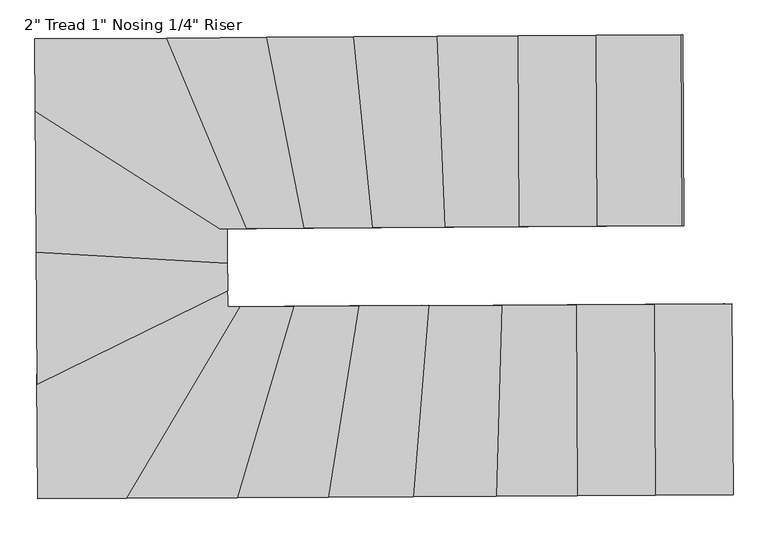
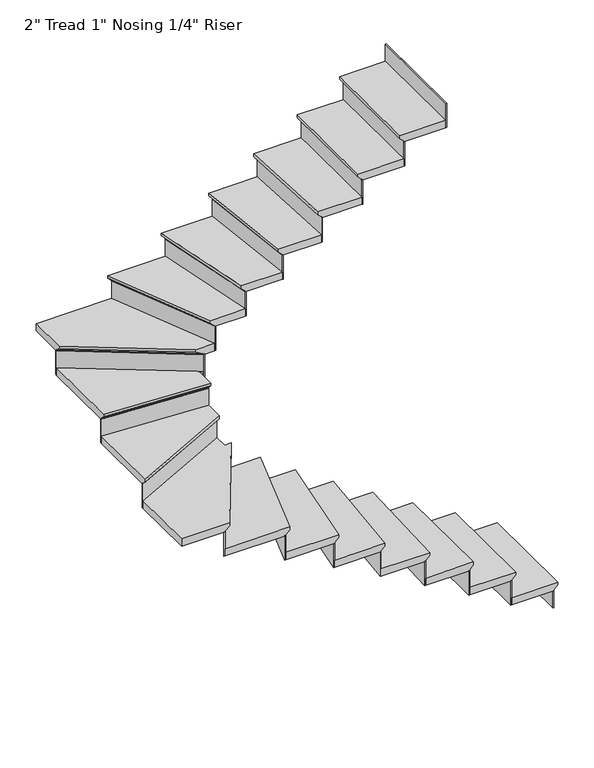
"""IFC4 building model written with IfcOpenShell, lengths in millimetres: stair flight geometry."""

from ifc_helpers import new_model, si_unit, origin, place, context, project, spatial, faceted_brep, source, transform, mapped, element, save


def stair_flight_c1b2dc12(model_context):
    return source(origin(), model_context, "Body", "Brep", [
        faceted_brep([(-120.6930289, -3539.621908, 12951.8833333), (-120.6930289, -3539.621908, 12970.9333333), (-116.4891496, -4225.4090232, 12970.9333333), (-116.4891496, -4225.4090232, 12951.8833333), (-146.0925517, -3539.7776072, 12926.4833333), (-141.8886723, -4225.5647224, 12926.4833333), (-425.4873024, -3541.4902988, 12970.9333333), (-421.283423, -4227.277414, 12970.9333333), (-141.8886723, -4225.5647224, 12920.1333333), (-421.283423, -4227.277414, 12920.1333333), (-425.4873024, -3541.4902988, 12920.1333333), (-146.0925517, -3539.7776072, 12920.1333333)], [[[0, 1, 2, 3]], [[4, 0, 3, 5]], [[2, 1, 6, 7]], [[8, 9, 10, 11]], [[2, 7, 9, 8, 5, 3]], [[8, 11, 4, 5]], [[6, 1, 0, 4, 11, 10]], [[7, 6, 10, 9]]]),
        faceted_brep([(-146.0925517, -3539.7776072, 12920.1333333), (-146.0925517, -3539.7776072, 12801.6), (-152.4424324, -3539.816532, 12801.6), (-152.4424324, -3539.816532, 12920.1333333), (-141.8886723, -4225.5647224, 12920.1333333), (-148.238553, -4225.6036472, 12920.1333333), (-148.238553, -4225.6036472, 12801.6), (-141.8886723, -4225.5647224, 12801.6)], [[[0, 1, 2, 3]], [[4, 5, 6, 7]], [[1, 0, 4, 7]], [[2, 1, 7, 6]], [[3, 2, 6, 5]], [[0, 3, 5, 4]]]),
        faceted_brep([(-425.4873024, -3541.4902988, 13089.4666667), (-425.4873024, -3541.4902988, 12920.1333333), (-431.8371831, -3541.5292236, 12920.1333333), (-431.8371831, -3541.5292236, 13089.4666667), (-421.283423, -4227.277414, 13089.4666667), (-427.6333037, -4227.3163388, 13089.4666667), (-427.6333037, -4227.3163388, 12920.1333333), (-421.283423, -4227.277414, 12920.1333333)], [[[0, 1, 2, 3]], [[4, 5, 6, 7]], [[1, 0, 4, 7]], [[2, 1, 7, 6]], [[3, 2, 6, 5]], [[0, 3, 5, 4]]]),
        faceted_brep([(-395.8839002, -4227.1217148, 13140.2666667), (-400.0877796, -3541.3345996, 13140.2666667), (-704.882053, -3543.2029904, 13140.2666667), (-700.6781736, -4228.9901056, 13140.2666667), (-421.283423, -4227.277414, 13089.4666667), (-700.6781736, -4228.9901056, 13089.4666667), (-704.882053, -3543.2029904, 13089.4666667), (-425.4873024, -3541.4902988, 13089.4666667), (-421.283423, -4227.277414, 13095.8166667), (-395.8839002, -4227.1217148, 13121.2166667), (-425.4873024, -3541.4902988, 13095.8166667), (-400.0877796, -3541.3345996, 13121.2166667)], [[[0, 1, 2, 3]], [[4, 5, 6, 7]], [[0, 3, 5, 4, 8, 9]], [[4, 7, 10, 8]], [[2, 1, 11, 10, 7, 6]], [[3, 2, 6, 5]], [[11, 1, 0, 9]], [[10, 11, 9, 8]]]),
        faceted_brep([(-704.882053, -3543.2029904, 13258.8), (-704.882053, -3543.2029904, 13089.4666667), (-711.2319337, -3543.2419152, 13089.4666667), (-711.2319337, -3543.2419152, 13258.8), (-700.6781736, -4228.9901056, 13258.8), (-707.0280543, -4229.0290304, 13258.8), (-707.0280543, -4229.0290304, 13089.4666667), (-700.6781736, -4228.9901056, 13089.4666667)], [[[0, 1, 2, 3]], [[4, 5, 6, 7]], [[1, 0, 4, 7]], [[2, 1, 7, 6]], [[3, 2, 6, 5]], [[0, 3, 5, 4]]]),
        faceted_brep([(-675.2786508, -4228.8344064, 13309.6), (-679.4825302, -3543.0472912, 13309.6), (-971.9344004, -3544.840023, 13309.6), (-992.4483132, -4230.7786584, 13309.6), (-700.6781736, -4228.9901056, 13258.8), (-992.4483132, -4230.7786584, 13258.8), (-971.9344004, -3544.840023, 13258.8), (-704.882053, -3543.2029904, 13258.8), (-700.6781736, -4228.9901056, 13265.15), (-675.2786508, -4228.8344064, 13290.55), (-704.882053, -3543.2029904, 13265.15), (-679.4825302, -3543.0472912, 13290.55)], [[[0, 1, 2, 3]], [[4, 5, 6, 7]], [[0, 3, 5, 4, 8, 9]], [[4, 7, 10, 8]], [[2, 1, 11, 10, 7, 6]], [[3, 2, 6, 5]], [[11, 1, 0, 9]], [[10, 11, 9, 8]]]),
        faceted_brep([(-971.9344004, -3544.840023, 13428.1333333), (-971.9344004, -3544.840023, 13258.8), (-978.2884043, -3544.8789731, 13258.8), (-978.2884043, -3544.8789731, 13428.1333333), (-992.4483132, -4230.7786584, 13428.1333333), (-998.8023171, -4230.8176085, 13428.1333333), (-998.8023171, -4230.8176085, 13258.8), (-992.4483132, -4230.7786584, 13258.8)], [[[0, 1, 2, 3]], [[4, 5, 6, 7]], [[1, 0, 4, 7]], [[2, 1, 7, 6]], [[3, 2, 6, 5]], [[0, 3, 5, 4]]]),
        faceted_brep([(-967.0322975, -4230.6228581, 13478.9333333), (-946.5183848, -3544.6842227, 13478.9333333), (-1233.842238, -3546.4455197, 13478.9333333), (-1289.4900883, -4232.5995264, 13478.9333333), (-992.4483132, -4230.7786584, 13428.1333333), (-1289.4900883, -4232.5995264, 13428.1333333), (-1233.842238, -3546.4455197, 13428.1333333), (-971.9344004, -3544.840023, 13428.1333333), (-992.4483132, -4230.7786584, 13434.4833333), (-967.0322975, -4230.6228581, 13459.8833333), (-971.9344004, -3544.840023, 13434.4833333), (-946.5183848, -3544.6842227, 13459.8833333)], [[[0, 1, 2, 3]], [[4, 5, 6, 7]], [[0, 3, 5, 4, 8, 9]], [[4, 7, 10, 8]], [[2, 1, 11, 10, 7, 6]], [[3, 2, 6, 5]], [[11, 1, 0, 9]], [[10, 11, 9, 8]]]),
        faceted_brep([(-1233.842238, -3546.4455197, 13597.4666667), (-1233.842238, -3546.4455197, 13428.1333333), (-1240.2162558, -3546.4845925, 13428.1333333), (-1240.2162558, -3546.4845925, 13597.4666667), (-1289.4900883, -4232.5995264, 13597.4666667), (-1295.8641061, -4232.6385992, 13597.4666667), (-1295.8641061, -4232.6385992, 13428.1333333), (-1289.4900883, -4232.5995264, 13428.1333333)], [[[0, 1, 2, 3]], [[4, 5, 6, 7]], [[1, 0, 4, 7]], [[2, 1, 7, 6]], [[3, 2, 6, 5]], [[0, 3, 5, 4]]]),
        faceted_brep([(-1263.994017, -4232.4432353, 13648.2666667), (-1208.3461666, -3546.2892286, 13648.2666667), (-1486.5415383, -3547.994568, 13648.2666667), (-1596.081167, -4234.4789317, 13648.2666667), (-1289.4900883, -4232.5995264, 13597.4666667), (-1596.081167, -4234.4789317, 13597.4666667), (-1486.5415383, -3547.994568, 13597.4666667), (-1233.842238, -3546.4455197, 13597.4666667), (-1289.4900883, -4232.5995264, 13603.8166667), (-1263.994017, -4232.4432353, 13629.2166667), (-1233.842238, -3546.4455197, 13603.8166667), (-1208.3461666, -3546.2892286, 13629.2166667)], [[[0, 1, 2, 3]], [[4, 5, 6, 7]], [[0, 3, 5, 4, 8, 9]], [[4, 7, 10, 8]], [[2, 1, 11, 10, 7, 6]], [[3, 2, 6, 5]], [[11, 1, 0, 9]], [[10, 11, 9, 8]]]),
        faceted_brep([(-1486.5415383, -3547.994568, 13766.8), (-1486.5415383, -3547.994568, 13597.4666667), (-1492.9781659, -3548.0340246, 13597.4666667), (-1492.9781659, -3548.0340246, 13766.8), (-1596.081167, -4234.4789317, 13766.8), (-1602.5177946, -4234.5183882, 13766.8), (-1602.5177946, -4234.5183882, 13597.4666667), (-1596.081167, -4234.4789317, 13597.4666667)], [[[0, 1, 2, 3]], [[4, 5, 6, 7]], [[1, 0, 4, 7]], [[2, 1, 7, 6]], [[3, 2, 6, 5]], [[0, 3, 5, 4]]]),
        faceted_brep([(-1570.3346568, -4234.3211054, 13817.6), (-1460.7950281, -3547.8367418, 13817.6), (-1720.1488607, -3549.4265824, 13817.6), (-1922.8306159, -4236.4819079, 13817.6), (-1596.081167, -4234.4789317, 13766.8), (-1922.8306159, -4236.4819079, 13766.8), (-1720.1488607, -3549.4265824, 13766.8), (-1486.5415383, -3547.994568, 13766.8), (-1596.081167, -4234.4789317, 13773.15), (-1570.3346568, -4234.3211054, 13798.55), (-1486.5415383, -3547.994568, 13773.15), (-1460.7950281, -3547.8367418, 13798.55)], [[[0, 1, 2, 3]], [[4, 5, 6, 7]], [[0, 3, 5, 4, 8, 9]], [[4, 7, 10, 8]], [[2, 1, 11, 10, 7, 6]], [[3, 2, 6, 5]], [[11, 1, 0, 9]], [[10, 11, 9, 8]]]),
        faceted_brep([(-1720.1488607, -3549.4265824, 13936.1333333), (-1720.1488607, -3549.4265824, 13766.8), (-1726.781397, -3549.4672399, 13766.8), (-1726.781397, -3549.4672399, 13936.1333333), (-1922.8306159, -4236.4819079, 13936.1333333), (-1929.4631522, -4236.5225654, 13936.1333333), (-1929.4631522, -4236.5225654, 13766.8), (-1922.8306159, -4236.4819079, 13766.8)], [[[0, 1, 2, 3]], [[4, 5, 6, 7]], [[1, 0, 4, 7]], [[2, 1, 7, 6]], [[3, 2, 6, 5]], [[0, 3, 5, 4]]]),
        faceted_brep([(-1896.3004707, -4236.3192779, 13986.9333333), (-1693.6187155, -3549.2639524, 13986.9333333), (-1917.3665941, -3550.6355283, 13986.9333333), (-2324.8688668, -4238.9464049, 13986.9333333), (-1922.8306159, -4236.4819079, 13936.1333333), (-2324.8688668, -4238.9464049, 13936.1333333), (-1917.3665941, -3550.6355283, 13936.1333333), (-1720.1488607, -3549.4265824, 13936.1333333), (-1922.8306159, -4236.4819079, 13942.4833333), (-1896.3004707, -4236.3192779, 13967.8833333), (-1720.1488607, -3549.4265824, 13942.4833333), (-1693.6187155, -3549.2639524, 13967.8833333)], [[[0, 1, 2, 3]], [[4, 5, 6, 7]], [[0, 3, 5, 4, 8, 9]], [[4, 7, 10, 8]], [[2, 1, 11, 10, 7, 6]], [[3, 2, 6, 5]], [[11, 1, 0, 9]], [[10, 11, 9, 8]]]),
        faceted_brep([(-1917.3665941, -3550.6355283, 14105.4666667), (-1917.3665941, -3550.6355283, 13936.1333333), (-1924.7728783, -3550.6809289, 13936.1333333), (-1924.7728783, -3550.6809289, 14105.4666667), (-2324.8688668, -4238.9464049, 14105.4666667), (-2332.275151, -4238.9918055, 14105.4666667), (-2332.275151, -4238.9918055, 13936.1333333), (-2324.8688668, -4238.9464049, 13936.1333333)], [[[0, 1, 2, 3]], [[4, 5, 6, 7]], [[1, 0, 4, 7]], [[2, 1, 7, 6]], [[3, 2, 6, 5]], [[0, 3, 5, 4]]]),
        faceted_brep([(-2615.3480869, -3801.2875551, 14156.2666667), (-2612.6544213, -4240.7105322, 14156.2666667), (-2295.24373, -4238.7648026, 14156.2666667), (-1887.7414574, -3550.4539261, 14156.2666667), (-1931.0711854, -3550.7195376, 14156.2666667), (-1931.5966592, -3464.9979706, 14156.2666667), (-2612.6544213, -4240.7105322, 14105.4666667), (-2615.3480869, -3801.2875551, 14105.4666667), (-1931.5966592, -3464.9979706, 14105.4666667), (-1931.0711854, -3550.7195376, 14105.4666667), (-1917.3665941, -3550.6355283, 14105.4666667), (-2324.8688668, -4238.9464049, 14105.4666667), (-1917.3665941, -3550.6355283, 14111.8166667), (-2324.8688668, -4238.9464049, 14111.8166667), (-1887.7414574, -3550.4539261, 14137.2166667), (-2295.24373, -4238.7648026, 14137.2166667)], [[[0, 1, 2, 3, 4, 5]], [[6, 7, 8, 9, 10, 11]], [[1, 0, 7, 6]], [[11, 10, 12, 13]], [[5, 4, 9, 8]], [[0, 5, 8, 7]], [[14, 3, 2, 15]], [[12, 14, 15, 13]], [[4, 3, 14, 12, 10, 9]], [[2, 1, 6, 11, 13, 15]]]),
        faceted_brep([(-1931.5966592, -3464.9979706, 14274.8), (-1931.5966592, -3464.9979706, 14105.4666667), (-1931.6399076, -3457.9427742, 14105.4666667), (-1931.6399076, -3457.9427742, 14274.8), (-2615.3480869, -3801.2875551, 14274.8), (-2615.3913353, -3794.2323587, 14274.8), (-2615.3913353, -3794.2323587, 14105.4666667), (-2615.3480869, -3801.2875551, 14105.4666667)], [[[0, 1, 2, 3]], [[4, 5, 6, 7]], [[1, 0, 4, 7]], [[2, 1, 7, 6]], [[3, 2, 6, 5]], [[0, 3, 5, 4]]]),
        faceted_brep([(-2615.1750933, -3829.5083406, 14325.6), (-1931.4236656, -3493.2187561, 14325.6), (-1932.1828972, -3369.3638122, 14325.6), (-2618.2387587, -3329.7265819, 14325.6), (-2615.3480869, -3801.2875551, 14274.8), (-2618.2387587, -3329.7265819, 14274.8), (-1932.1828972, -3369.3638122, 14274.8), (-1931.5966592, -3464.9979706, 14274.8), (-2615.3480869, -3801.2875551, 14281.15), (-2615.1750933, -3829.5083406, 14306.55), (-1931.5966592, -3464.9979706, 14281.15), (-1931.4236656, -3493.2187561, 14306.55)], [[[0, 1, 2, 3]], [[4, 5, 6, 7]], [[0, 3, 5, 4, 8, 9]], [[4, 7, 10, 8]], [[2, 1, 11, 10, 7, 6]], [[3, 2, 6, 5]], [[11, 1, 0, 9]], [[10, 11, 9, 8]]]),
        faceted_brep([(-1932.1828972, -3369.3638122, 14444.1333333), (-1932.1828972, -3369.3638122, 14274.8), (-1932.2219015, -3363.0009693, 14274.8), (-1932.2219015, -3363.0009693, 14444.1333333), (-2618.2387587, -3329.7265819, 14444.1333333), (-2618.277763, -3323.363739, 14444.1333333), (-2618.277763, -3323.363739, 14274.8), (-2618.2387587, -3329.7265819, 14274.8)], [[[0, 1, 2, 3]], [[4, 5, 6, 7]], [[1, 0, 4, 7]], [[2, 1, 7, 6]], [[3, 2, 6, 5]], [[0, 3, 5, 4]]]),
        faceted_brep([(-2618.0827416, -3355.1779533, 14494.9333333), (-1932.0268801, -3394.8151835, 14494.9333333), (-1932.783877, -3271.3247869, 14494.9333333), (-1912.0496222, -3271.1976858, 14494.9333333), (-2621.364296, -2819.8515342, 14494.9333333), (-2618.2387587, -3329.7265819, 14444.1333333), (-2621.364296, -2819.8515342, 14444.1333333), (-1912.0496222, -3271.1976858, 14444.1333333), (-1932.783877, -3271.3247869, 14444.1333333), (-1932.1828972, -3369.3638122, 14444.1333333), (-2618.2387587, -3329.7265819, 14450.4833333), (-2618.0827416, -3355.1779533, 14475.8833333), (-1932.1828972, -3369.3638122, 14450.4833333), (-1932.0268801, -3394.8151835, 14475.8833333)], [[[0, 1, 2, 3, 4]], [[5, 6, 7, 8, 9]], [[0, 4, 6, 5, 10, 11]], [[5, 9, 12, 10]], [[2, 1, 13, 12, 9, 8]], [[3, 2, 8, 7]], [[4, 3, 7, 6]], [[13, 1, 0, 11]], [[12, 13, 11, 10]]]),
        faceted_brep([(-1912.0496222, -3271.1976858, 14613.4666667), (-1912.0496222, -3271.1976858, 14444.1333333), (-1900.3341194, -3271.1258697, 14444.1333333), (-1900.3341194, -3271.1258697, 14613.4666667), (-2621.364296, -2819.8515342, 14613.4666667), (-2621.4106144, -2812.2955182, 14613.4666667), (-2621.4106144, -2812.2955182, 14444.1333333), (-2621.364296, -2819.8515342, 14444.1333333)], [[[0, 1, 2, 3]], [[4, 5, 6, 7]], [[1, 0, 4, 7]], [[2, 1, 7, 6]], [[3, 2, 6, 5]], [[0, 3, 5, 4]]]),
        faceted_brep([(-2121.4312205, -2586.6683113, 14664.2666667), (-2622.7748716, -2589.7415511, 14664.2666667), (-2621.1790223, -2850.0755978, 14664.2666667), (-1958.9116334, -3271.4849502, 14664.2666667), (-1835.3232791, -3270.7273529, 14664.2666667), (-2622.7748716, -2589.7415511, 14613.4666667), (-2121.4312205, -2586.6683113, 14613.4666667), (-1835.3232791, -3270.7273529, 14613.4666667), (-1912.0496222, -3271.1976858, 14613.4666667), (-2621.364296, -2819.8515342, 14613.4666667), (-2621.364296, -2819.8515342, 14619.8166667), (-2621.1790223, -2850.0755978, 14645.2166667), (-1912.0496222, -3271.1976858, 14619.8166667), (-1958.9116334, -3271.4849502, 14645.2166667)], [[[0, 1, 2, 3, 4]], [[5, 6, 7, 8, 9]], [[1, 0, 6, 5]], [[2, 1, 5, 9, 10, 11]], [[9, 8, 12, 10]], [[0, 4, 7, 6]], [[13, 3, 2, 11]], [[12, 13, 11, 10]], [[4, 3, 13, 12, 8, 7]]]),
        faceted_brep([(-1835.3232791, -3270.7273529, 14782.8), (-1835.3232791, -3270.7273529, 14613.4666667), (-1828.4578405, -3270.6852677, 14613.4666667), (-1828.4578405, -3270.6852677, 14782.8), (-2121.4312205, -2586.6683113, 14782.8), (-2114.5657819, -2586.6262261, 14782.8), (-2114.5657819, -2586.6262261, 14613.4666667), (-2121.4312205, -2586.6683113, 14613.4666667)], [[[0, 1, 2, 3]], [[4, 5, 6, 7]], [[1, 0, 4, 7]], [[2, 1, 7, 6]], [[3, 2, 6, 5]], [[0, 3, 5, 4]]]),
        faceted_brep([(-2148.8929752, -2586.8366521, 14833.6), (-1862.7850338, -3270.8956936, 14833.6), (-1630.6514822, -3269.4727134, 14833.6), (-1765.0751589, -2584.4838464, 14833.6), (-2121.4312205, -2586.6683113, 14782.8), (-1765.0751589, -2584.4838464, 14782.8), (-1630.6514822, -3269.4727134, 14782.8), (-1835.3232791, -3270.7273529, 14782.8), (-2121.4312205, -2586.6683113, 14789.15), (-2148.8929752, -2586.8366521, 14814.55), (-1835.3232791, -3270.7273529, 14789.15), (-1862.7850338, -3270.8956936, 14814.55)], [[[0, 1, 2, 3]], [[4, 5, 6, 7]], [[0, 3, 5, 4, 8, 9]], [[4, 7, 10, 8]], [[2, 1, 11, 10, 7, 6]], [[3, 2, 6, 5]], [[11, 1, 0, 9]], [[10, 11, 9, 8]]]),
        faceted_brep([(-1630.6514822, -3269.4727134, 14952.1333333), (-1630.6514822, -3269.4727134, 14782.8), (-1624.1881401, -3269.4330931, 14782.8), (-1624.1881401, -3269.4330931, 14952.1333333), (-1765.0751589, -2584.4838464, 14952.1333333), (-1758.6118168, -2584.4442261, 14952.1333333), (-1758.6118168, -2584.4442261, 14782.8), (-1765.0751589, -2584.4838464, 14782.8)], [[[0, 1, 2, 3]], [[4, 5, 6, 7]], [[1, 0, 4, 7]], [[2, 1, 7, 6]], [[3, 2, 6, 5]], [[0, 3, 5, 4]]]),
        faceted_brep([(-1790.9285273, -2584.6423277, 15002.9333333), (-1656.5048506, -3269.6311948, 15002.9333333), (-1385.319119, -3267.9688245, 15002.9333333), (-1452.3132293, -2582.5666138, 15002.9333333), (-1765.0751589, -2584.4838464, 14952.1333333), (-1452.3132293, -2582.5666138, 14952.1333333), (-1385.319119, -3267.9688245, 14952.1333333), (-1630.6514822, -3269.4727134, 14952.1333333), (-1765.0751589, -2584.4838464, 14958.4833333), (-1790.9285273, -2584.6423277, 14983.8833333), (-1630.6514822, -3269.4727134, 14958.4833333), (-1656.5048506, -3269.6311948, 14983.8833333)], [[[0, 1, 2, 3]], [[4, 5, 6, 7]], [[0, 3, 5, 4, 8, 9]], [[4, 7, 10, 8]], [[2, 1, 11, 10, 7, 6]], [[3, 2, 6, 5]], [[11, 1, 0, 9]], [[10, 11, 9, 8]]]),
        faceted_brep([(-1385.319119, -3267.9688245, 15121.4666667), (-1385.319119, -3267.9688245, 14952.1333333), (-1378.942678, -3267.9297369, 14952.1333333), (-1378.942678, -3267.9297369, 15121.4666667), (-1452.3132293, -2582.5666138, 15121.4666667), (-1445.9367882, -2582.5275262, 15121.4666667), (-1445.9367882, -2582.5275262, 14952.1333333), (-1452.3132293, -2582.5666138, 14952.1333333)], [[[0, 1, 2, 3]], [[4, 5, 6, 7]], [[1, 0, 4, 7]], [[2, 1, 7, 6]], [[3, 2, 6, 5]], [[0, 3, 5, 4]]]),
        faceted_brep([(-1477.8189934, -2582.7229643, 15172.2666667), (-1410.8248832, -3268.125175, 15172.2666667), (-1125.1141805, -3266.3737666, 15172.2666667), (-1153.9085026, -2580.7373909, 15172.2666667), (-1452.3132293, -2582.5666138, 15121.4666667), (-1153.9085026, -2580.7373909, 15121.4666667), (-1125.1141805, -3266.3737666, 15121.4666667), (-1385.319119, -3267.9688245, 15121.4666667), (-1452.3132293, -2582.5666138, 15127.8166667), (-1477.8189934, -2582.7229643, 15153.2166667), (-1385.319119, -3267.9688245, 15127.8166667), (-1410.8248832, -3268.125175, 15153.2166667)], [[[0, 1, 2, 3]], [[4, 5, 6, 7]], [[0, 3, 5, 4, 8, 9]], [[4, 7, 10, 8]], [[2, 1, 11, 10, 7, 6]], [[3, 2, 6, 5]], [[11, 1, 0, 9]], [[10, 11, 9, 8]]]),
        faceted_brep([(-1125.1141805, -3266.3737666, 15290.8), (-1125.1141805, -3266.3737666, 15121.4666667), (-1118.7602189, -3266.3348167, 15121.4666667), (-1118.7602189, -3266.3348167, 15290.8), (-1153.9085026, -2580.7373909, 15290.8), (-1147.554541, -2580.6984411, 15290.8), (-1147.554541, -2580.6984411, 15121.4666667), (-1153.9085026, -2580.7373909, 15121.4666667)], [[[0, 1, 2, 3]], [[4, 5, 6, 7]], [[1, 0, 4, 7]], [[2, 1, 7, 6]], [[3, 2, 6, 5]], [[0, 3, 5, 4]]]),
        faceted_brep([(-1179.3243487, -2580.8931902, 15341.6), (-1150.5300267, -3266.5295659, 15341.6), (-858.0309746, -3264.7365448, 15341.6), (-862.2348539, -2578.9494296, 15341.6), (-1153.9085026, -2580.7373909, 15290.8), (-862.2348539, -2578.9494296, 15290.8), (-858.0309746, -3264.7365448, 15290.8), (-1125.1141805, -3266.3737666, 15290.8), (-1153.9085026, -2580.7373909, 15297.15), (-1179.3243487, -2580.8931902, 15322.55), (-1125.1141805, -3266.3737666, 15297.15), (-1150.5300267, -3266.5295659, 15322.55)], [[[0, 1, 2, 3]], [[4, 5, 6, 7]], [[0, 3, 5, 4, 8, 9]], [[4, 7, 10, 8]], [[2, 1, 11, 10, 7, 6]], [[3, 2, 6, 5]], [[11, 1, 0, 9]], [[10, 11, 9, 8]]]),
        faceted_brep([(-858.0309746, -3264.7365448, 15460.1333333), (-858.0309746, -3264.7365448, 15290.8), (-851.6810939, -3264.69762, 15290.8), (-851.6810939, -3264.69762, 15460.1333333), (-862.2348539, -2578.9494296, 15460.1333333), (-855.8849733, -2578.9105048, 15460.1333333), (-855.8849733, -2578.9105048, 15290.8), (-862.2348539, -2578.9494296, 15290.8)], [[[0, 1, 2, 3]], [[4, 5, 6, 7]], [[1, 0, 4, 7]], [[2, 1, 7, 6]], [[3, 2, 6, 5]], [[0, 3, 5, 4]]]),
        faceted_brep([(-887.6343767, -2579.1051288, 15510.9333333), (-883.4304974, -3264.8922441, 15510.9333333), (-578.6362239, -3263.0238532, 15510.9333333), (-582.8401033, -2577.236738, 15510.9333333), (-862.2348539, -2578.9494296, 15460.1333333), (-582.8401033, -2577.236738, 15460.1333333), (-578.6362239, -3263.0238532, 15460.1333333), (-858.0309746, -3264.7365448, 15460.1333333), (-862.2348539, -2578.9494296, 15466.4833333), (-887.6343767, -2579.1051288, 15491.8833333), (-858.0309746, -3264.7365448, 15466.4833333), (-883.4304974, -3264.8922441, 15491.8833333)], [[[0, 1, 2, 3]], [[4, 5, 6, 7]], [[0, 3, 5, 4, 8, 9]], [[4, 7, 10, 8]], [[2, 1, 11, 10, 7, 6]], [[3, 2, 6, 5]], [[11, 1, 0, 9]], [[10, 11, 9, 8]]]),
        faceted_brep([(-578.6362239, -3263.0238532, 15629.4666667), (-578.6362239, -3263.0238532, 15460.1333333), (-572.2863432, -3262.9849284, 15460.1333333), (-572.2863432, -3262.9849284, 15629.4666667), (-582.8401033, -2577.236738, 15629.4666667), (-576.4902226, -2577.1978132, 15629.4666667), (-576.4902226, -2577.1978132, 15460.1333333), (-582.8401033, -2577.236738, 15460.1333333)], [[[0, 1, 2, 3]], [[4, 5, 6, 7]], [[1, 0, 4, 7]], [[2, 1, 7, 6]], [[3, 2, 6, 5]], [[0, 3, 5, 4]]]),
        faceted_brep([(-299.2414733, -3261.3111616, 15798.8), (-299.2414733, -3261.3111616, 15629.4666667), (-292.8915926, -3261.2722368, 15629.4666667), (-292.8915926, -3261.2722368, 15798.8), (-303.4453527, -2575.5240464, 15798.8), (-297.095472, -2575.4851216, 15798.8), (-297.095472, -2575.4851216, 15629.4666667), (-303.4453527, -2575.5240464, 15629.4666667)], [[[0, 1, 2, 3]], [[4, 5, 6, 7]], [[1, 0, 4, 7]], [[2, 1, 7, 6]], [[3, 2, 6, 5]], [[0, 3, 5, 4]]]),
        faceted_brep([(-608.2396261, -2577.3924372, 15680.2666667), (-604.0357467, -3263.1795525, 15680.2666667), (-299.2414733, -3261.3111616, 15680.2666667), (-303.4453527, -2575.5240464, 15680.2666667), (-582.8401033, -2577.236738, 15629.4666667), (-303.4453527, -2575.5240464, 15629.4666667), (-299.2414733, -3261.3111616, 15629.4666667), (-578.6362239, -3263.0238532, 15629.4666667), (-582.8401033, -2577.236738, 15635.8166667), (-608.2396261, -2577.3924372, 15661.2166667), (-578.6362239, -3263.0238532, 15635.8166667), (-604.0357467, -3263.1795525, 15661.2166667)], [[[0, 1, 2, 3]], [[4, 5, 6, 7]], [[0, 3, 5, 4, 8, 9]], [[4, 7, 10, 8]], [[2, 1, 11, 10, 7, 6]], [[3, 2, 6, 5]], [[11, 1, 0, 9]], [[10, 11, 9, 8]]]),
    ])


if __name__ == "__main__":
    model = new_model("IFC4")
    model_context = context("Model", 3, world=origin())
    ifc_project = project(units=[si_unit("LENGTHUNIT", "METRE", prefix="MILLI")], contexts=[model_context])
    site = spatial("IfcSite", under=ifc_project)
    building = spatial("IfcBuilding", under=site)
    placement = place(None, origin())
    stair_flight_shape = stair_flight_c1b2dc12(model_context)
    element("IfcStairFlight", 1, ObjectType="2\" Tread 1\" Nosing 1/4\" Riser", at=placement, inside=building, context=model_context, shape_type="MappedRepresentation", body=[
        mapped(stair_flight_shape, transform((0.0, 0.0, 0.0), x_axis=(1.0, 0.0, 0.0), y_axis=(0.0, 1.0, 0.0), z_axis=(0.0, 0.0, 1.0))),
    ])
    save(model, "model.ifc")
